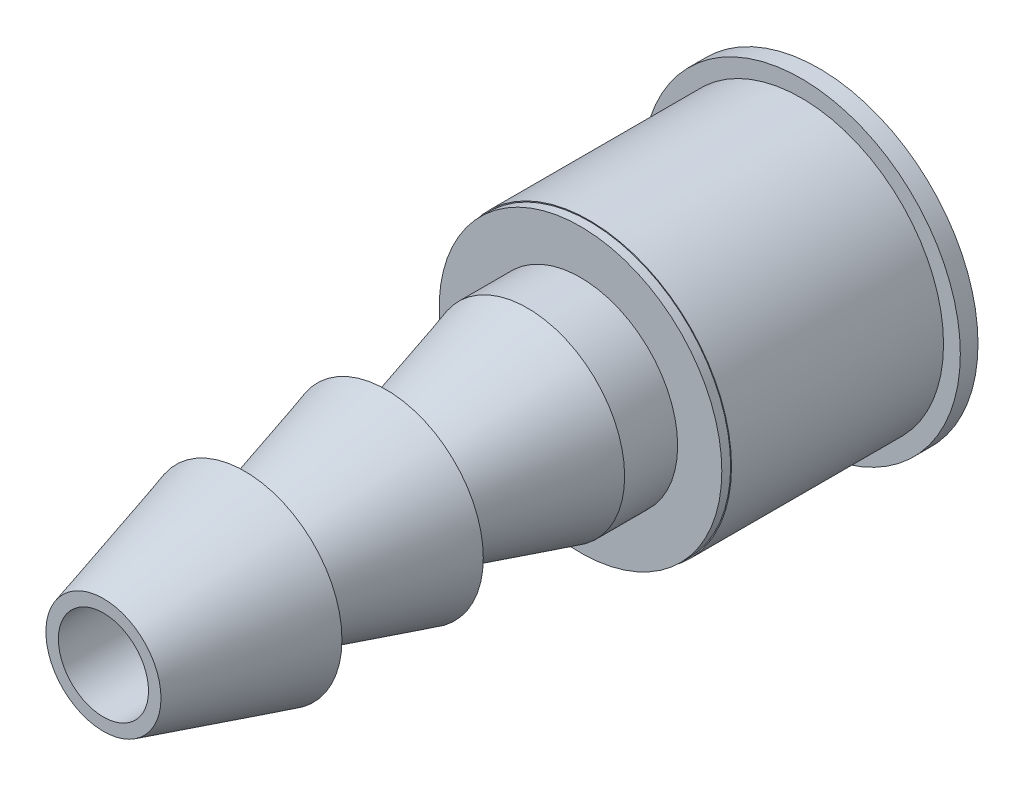
ISO-10303-21;
HEADER;
FILE_DESCRIPTION(('STEP AP214'),'2;1');
FILE_NAME('part.step','',(''),(''),'','','');
FILE_SCHEMA(('AUTOMOTIVE_DESIGN { 1 0 10303 214 1 1 1 1 }'));
ENDSEC;
DATA;
#1=APPLICATION_CONTEXT('core data for automotive mechanical design processes');
#2=APPLICATION_PROTOCOL_DEFINITION('international standard','automotive_design',2000,#1);
#3=PRODUCT_CONTEXT('',#1,'mechanical');
#4=PRODUCT('Part','Part','',(#3));
#5=PRODUCT_RELATED_PRODUCT_CATEGORY('part','',(#4));
#6=PRODUCT_DEFINITION_FORMATION('','',#4);
#7=PRODUCT_DEFINITION_CONTEXT('part definition',#1,'design');
#8=PRODUCT_DEFINITION('design','',#6,#7);
#9=PRODUCT_DEFINITION_SHAPE('','',#8);
#10=(LENGTH_UNIT() NAMED_UNIT(*) SI_UNIT(.MILLI.,.METRE.));
#11=(NAMED_UNIT(*) PLANE_ANGLE_UNIT() SI_UNIT($,.RADIAN.));
#12=(NAMED_UNIT(*) SI_UNIT($,.STERADIAN.) SOLID_ANGLE_UNIT());
#13=UNCERTAINTY_MEASURE_WITH_UNIT(LENGTH_MEASURE(1.E-05),#10,'distance_accuracy_value','');
#14=(GEOMETRIC_REPRESENTATION_CONTEXT(3) GLOBAL_UNCERTAINTY_ASSIGNED_CONTEXT((#13)) GLOBAL_UNIT_ASSIGNED_CONTEXT((#10,
#11,#12)) REPRESENTATION_CONTEXT('',''));
#15=CARTESIAN_POINT('',(0.,0.,0.));
#16=DIRECTION('',(0.,0.,1.));
#17=DIRECTION('',(1.,0.,0.));
#18=AXIS2_PLACEMENT_3D('',#15,#16,#17);
#19=CARTESIAN_POINT('',(0.,0.,1.));
#20=DIRECTION('',(0.,0.,-1.));
#21=DIRECTION('',(-1.,0.,0.));
#22=AXIS2_PLACEMENT_3D('',#19,#20,#21);
#23=CYLINDRICAL_SURFACE('',#22,9.);
#24=CARTESIAN_POINT('',(0.,0.,1.));
#25=DIRECTION('',(0.,0.,1.));
#26=DIRECTION('',(1.,0.,0.));
#27=AXIS2_PLACEMENT_3D('',#24,#25,#26);
#28=CIRCLE('',#27,9.);
#29=CARTESIAN_POINT('',(9.,0.,1.));
#30=VERTEX_POINT('',#29);
#31=EDGE_CURVE('E66',#30,#30,#28,.T.);
#32=ORIENTED_EDGE('',*,*,#31,.F.);
#33=EDGE_LOOP('',(#32));
#34=FACE_BOUND('',#33,.T.);
#35=CARTESIAN_POINT('',(0.,0.,0.));
#36=DIRECTION('',(0.,0.,1.));
#37=DIRECTION('',(1.,0.,0.));
#38=AXIS2_PLACEMENT_3D('',#35,#36,#37);
#39=CIRCLE('',#38,9.);
#40=CARTESIAN_POINT('',(9.,0.,0.));
#41=VERTEX_POINT('',#40);
#42=EDGE_CURVE('E70',#41,#41,#39,.T.);
#43=ORIENTED_EDGE('',*,*,#42,.T.);
#44=EDGE_LOOP('',(#43));
#45=FACE_BOUND('',#44,.T.);
#46=ADVANCED_FACE('F43',(#34,#45),#23,.T.);
#47=CARTESIAN_POINT('',(0.,0.,1.));
#48=DIRECTION('',(0.,0.,1.));
#49=DIRECTION('',(1.,0.,0.));
#50=AXIS2_PLACEMENT_3D('',#47,#48,#49);
#51=PLANE('',#50);
#52=CARTESIAN_POINT('',(0.,0.,1.));
#53=DIRECTION('',(0.,0.,1.));
#54=DIRECTION('',(1.,0.,0.));
#55=AXIS2_PLACEMENT_3D('',#52,#53,#54);
#56=CIRCLE('',#55,8.05);
#57=CARTESIAN_POINT('',(8.05,0.,1.));
#58=VERTEX_POINT('',#57);
#59=EDGE_CURVE('E54',#58,#58,#56,.T.);
#60=ORIENTED_EDGE('',*,*,#59,.F.);
#61=EDGE_LOOP('',(#60));
#62=FACE_BOUND('',#61,.T.);
#63=ORIENTED_EDGE('',*,*,#31,.T.);
#64=EDGE_LOOP('',(#63));
#65=FACE_BOUND('',#64,.T.);
#66=ADVANCED_FACE('F79',(#62,#65),#51,.T.);
#67=CARTESIAN_POINT('',(0.,0.,0.));
#68=DIRECTION('',(0.,0.,1.));
#69=DIRECTION('',(1.,0.,0.));
#70=AXIS2_PLACEMENT_3D('',#67,#68,#69);
#71=PLANE('',#70);
#72=CARTESIAN_POINT('',(0.,0.,0.));
#73=DIRECTION('',(0.,0.,-1.));
#74=DIRECTION('',(-1.,0.,0.));
#75=AXIS2_PLACEMENT_3D('',#72,#73,#74);
#76=CIRCLE('',#75,5.5);
#77=CARTESIAN_POINT('',(-5.5,0.,0.));
#78=VERTEX_POINT('',#77);
#79=EDGE_CURVE('E351',#78,#78,#76,.T.);
#80=ORIENTED_EDGE('',*,*,#79,.F.);
#81=EDGE_LOOP('',(#80));
#82=FACE_BOUND('',#81,.T.);
#83=ORIENTED_EDGE('',*,*,#42,.F.);
#84=EDGE_LOOP('',(#83));
#85=FACE_BOUND('',#84,.T.);
#86=ADVANCED_FACE('F77',(#82,#85),#71,.F.);
#87=CARTESIAN_POINT('',(0.,0.,13.));
#88=DIRECTION('',(0.,0.,-1.));
#89=DIRECTION('',(-1.,0.,0.));
#90=AXIS2_PLACEMENT_3D('',#87,#88,#89);
#91=CYLINDRICAL_SURFACE('',#90,8.05);
#92=CARTESIAN_POINT('',(0.,0.,13.));
#93=DIRECTION('',(0.,0.,1.));
#94=DIRECTION('',(1.,0.,0.));
#95=AXIS2_PLACEMENT_3D('',#92,#93,#94);
#96=CIRCLE('',#95,8.05);
#97=CARTESIAN_POINT('',(8.05,0.,13.));
#98=VERTEX_POINT('',#97);
#99=EDGE_CURVE('E65',#98,#98,#96,.T.);
#100=ORIENTED_EDGE('',*,*,#99,.F.);
#101=EDGE_LOOP('',(#100));
#102=FACE_BOUND('',#101,.T.);
#103=ORIENTED_EDGE('',*,*,#59,.T.);
#104=EDGE_LOOP('',(#103));
#105=FACE_BOUND('',#104,.T.);
#106=ADVANCED_FACE('F76',(#102,#105),#91,.T.);
#107=CARTESIAN_POINT('',(0.,0.,13.));
#108=DIRECTION('',(0.,0.,1.));
#109=DIRECTION('',(1.,0.,0.));
#110=AXIS2_PLACEMENT_3D('',#107,#108,#109);
#111=PLANE('',#110);
#112=CARTESIAN_POINT('',(0.,0.,13.));
#113=DIRECTION('',(0.,0.,1.));
#114=DIRECTION('',(1.,0.,0.));
#115=AXIS2_PLACEMENT_3D('',#112,#113,#114);
#116=CIRCLE('',#115,8.);
#117=CARTESIAN_POINT('',(8.,0.,13.));
#118=VERTEX_POINT('',#117);
#119=EDGE_CURVE('E49',#118,#118,#116,.T.);
#120=ORIENTED_EDGE('',*,*,#119,.F.);
#121=EDGE_LOOP('',(#120));
#122=FACE_BOUND('',#121,.T.);
#123=ORIENTED_EDGE('',*,*,#99,.T.);
#124=EDGE_LOOP('',(#123));
#125=FACE_BOUND('',#124,.T.);
#126=ADVANCED_FACE('F82',(#122,#125),#111,.T.);
#127=CARTESIAN_POINT('',(0.,0.,13.5));
#128=DIRECTION('',(0.,0.,-1.));
#129=DIRECTION('',(-1.,0.,0.));
#130=AXIS2_PLACEMENT_3D('',#127,#128,#129);
#131=CYLINDRICAL_SURFACE('',#130,8.);
#132=CARTESIAN_POINT('',(0.,0.,13.5));
#133=DIRECTION('',(0.,0.,1.));
#134=DIRECTION('',(1.,0.,0.));
#135=AXIS2_PLACEMENT_3D('',#132,#133,#134);
#136=CIRCLE('',#135,8.);
#137=CARTESIAN_POINT('',(8.,0.,13.5));
#138=VERTEX_POINT('',#137);
#139=EDGE_CURVE('E64',#138,#138,#136,.T.);
#140=ORIENTED_EDGE('',*,*,#139,.F.);
#141=EDGE_LOOP('',(#140));
#142=FACE_BOUND('',#141,.T.);
#143=ORIENTED_EDGE('',*,*,#119,.T.);
#144=EDGE_LOOP('',(#143));
#145=FACE_BOUND('',#144,.T.);
#146=ADVANCED_FACE('F124',(#142,#145),#131,.T.);
#147=CARTESIAN_POINT('',(0.,0.,13.5));
#148=DIRECTION('',(0.,0.,1.));
#149=DIRECTION('',(1.,0.,0.));
#150=AXIS2_PLACEMENT_3D('',#147,#148,#149);
#151=PLANE('',#150);
#152=CARTESIAN_POINT('',(0.,0.,13.5));
#153=DIRECTION('',(0.,0.,1.));
#154=DIRECTION('',(1.,0.,0.));
#155=AXIS2_PLACEMENT_3D('',#152,#153,#154);
#156=CIRCLE('',#155,5.5);
#157=CARTESIAN_POINT('',(5.5,0.,13.5));
#158=VERTEX_POINT('',#157);
#159=EDGE_CURVE('E10',#158,#158,#156,.T.);
#160=ORIENTED_EDGE('',*,*,#159,.F.);
#161=EDGE_LOOP('',(#160));
#162=FACE_BOUND('',#161,.T.);
#163=ORIENTED_EDGE('',*,*,#139,.T.);
#164=EDGE_LOOP('',(#163));
#165=FACE_BOUND('',#164,.T.);
#166=ADVANCED_FACE('F133',(#162,#165),#151,.T.);
#167=CARTESIAN_POINT('',(0.,0.,16.5));
#168=DIRECTION('',(0.,0.,-1.));
#169=DIRECTION('',(-1.,0.,0.));
#170=AXIS2_PLACEMENT_3D('',#167,#168,#169);
#171=CYLINDRICAL_SURFACE('',#170,5.5);
#172=CARTESIAN_POINT('',(0.,0.,16.5));
#173=DIRECTION('',(0.,0.,1.));
#174=DIRECTION('',(1.,0.,0.));
#175=AXIS2_PLACEMENT_3D('',#172,#173,#174);
#176=CIRCLE('',#175,5.5);
#177=CARTESIAN_POINT('',(5.5,0.,16.5));
#178=VERTEX_POINT('',#177);
#179=EDGE_CURVE('E56',#178,#178,#176,.T.);
#180=ORIENTED_EDGE('',*,*,#179,.F.);
#181=EDGE_LOOP('',(#180));
#182=FACE_BOUND('',#181,.T.);
#183=ORIENTED_EDGE('',*,*,#159,.T.);
#184=EDGE_LOOP('',(#183));
#185=FACE_BOUND('',#184,.T.);
#186=ADVANCED_FACE('F141',(#182,#185),#171,.T.);
#187=CARTESIAN_POINT('',(0.,0.,16.5));
#188=DIRECTION('',(0.,0.,-1.));
#189=DIRECTION('',(1.,0.,0.));
#190=AXIS2_PLACEMENT_3D('',#187,#188,#189);
#191=CONICAL_SURFACE('',#190,5.5,0.273318560862313);
#192=CARTESIAN_POINT('',(0.,0.,24.5));
#193=DIRECTION('',(0.,0.,1.));
#194=DIRECTION('',(1.,0.,0.));
#195=AXIS2_PLACEMENT_3D('',#192,#193,#194);
#196=CIRCLE('',#195,3.25732656296489);
#197=CARTESIAN_POINT('',(3.25732656296489,0.,24.5));
#198=VERTEX_POINT('',#197);
#199=EDGE_CURVE('E373',#198,#198,#196,.T.);
#200=ORIENTED_EDGE('',*,*,#199,.F.);
#201=EDGE_LOOP('',(#200));
#202=FACE_BOUND('',#201,.T.);
#203=ORIENTED_EDGE('',*,*,#179,.T.);
#204=EDGE_LOOP('',(#203));
#205=FACE_BOUND('',#204,.T.);
#206=ADVANCED_FACE('F153',(#202,#205),#191,.T.);
#207=CARTESIAN_POINT('',(0.,0.,24.5));
#208=DIRECTION('',(0.,0.,-1.));
#209=DIRECTION('',(1.,0.,0.));
#210=AXIS2_PLACEMENT_3D('',#207,#208,#209);
#211=CONICAL_SURFACE('',#210,5.5,0.273318560862313);
#212=CARTESIAN_POINT('',(0.,0.,32.5));
#213=DIRECTION('',(0.,0.,1.));
#214=DIRECTION('',(1.,0.,0.));
#215=AXIS2_PLACEMENT_3D('',#212,#213,#214);
#216=CIRCLE('',#215,3.25732656296489);
#217=CARTESIAN_POINT('',(3.25732656296489,0.,32.5));
#218=VERTEX_POINT('',#217);
#219=EDGE_CURVE('E371',#218,#218,#216,.T.);
#220=ORIENTED_EDGE('',*,*,#219,.F.);
#221=EDGE_LOOP('',(#220));
#222=FACE_BOUND('',#221,.T.);
#223=CARTESIAN_POINT('',(0.,0.,24.5));
#224=DIRECTION('',(0.,0.,1.));
#225=DIRECTION('',(1.,0.,0.));
#226=AXIS2_PLACEMENT_3D('',#223,#224,#225);
#227=CIRCLE('',#226,5.5);
#228=CARTESIAN_POINT('',(5.5,0.,24.5));
#229=VERTEX_POINT('',#228);
#230=EDGE_CURVE('E368',#229,#229,#227,.T.);
#231=ORIENTED_EDGE('',*,*,#230,.T.);
#232=EDGE_LOOP('',(#231));
#233=FACE_BOUND('',#232,.T.);
#234=ADVANCED_FACE('F162',(#222,#233),#211,.T.);
#235=CARTESIAN_POINT('',(0.,0.,24.5));
#236=DIRECTION('',(0.,0.,1.));
#237=DIRECTION('',(1.,0.,0.));
#238=AXIS2_PLACEMENT_3D('',#235,#236,#237);
#239=PLANE('',#238);
#240=ORIENTED_EDGE('',*,*,#199,.T.);
#241=EDGE_LOOP('',(#240));
#242=FACE_BOUND('',#241,.T.);
#243=ORIENTED_EDGE('',*,*,#230,.F.);
#244=EDGE_LOOP('',(#243));
#245=FACE_BOUND('',#244,.T.);
#246=ADVANCED_FACE('F175',(#242,#245),#239,.F.);
#247=CARTESIAN_POINT('',(0.,0.,32.5));
#248=DIRECTION('',(0.,0.,-1.));
#249=DIRECTION('',(1.,0.,0.));
#250=AXIS2_PLACEMENT_3D('',#247,#248,#249);
#251=CONICAL_SURFACE('',#250,5.5,0.273318560862313);
#252=CARTESIAN_POINT('',(0.,0.,40.5));
#253=DIRECTION('',(0.,0.,1.));
#254=DIRECTION('',(1.,0.,0.));
#255=AXIS2_PLACEMENT_3D('',#252,#253,#254);
#256=CIRCLE('',#255,3.25732656296489);
#257=CARTESIAN_POINT('',(3.25732656296489,0.,40.5));
#258=VERTEX_POINT('',#257);
#259=EDGE_CURVE('E362',#258,#258,#256,.T.);
#260=ORIENTED_EDGE('',*,*,#259,.F.);
#261=EDGE_LOOP('',(#260));
#262=FACE_BOUND('',#261,.T.);
#263=CARTESIAN_POINT('',(0.,0.,32.5));
#264=DIRECTION('',(0.,0.,1.));
#265=DIRECTION('',(1.,0.,0.));
#266=AXIS2_PLACEMENT_3D('',#263,#264,#265);
#267=CIRCLE('',#266,5.5);
#268=CARTESIAN_POINT('',(5.5,0.,32.5));
#269=VERTEX_POINT('',#268);
#270=EDGE_CURVE('E359',#269,#269,#267,.T.);
#271=ORIENTED_EDGE('',*,*,#270,.T.);
#272=EDGE_LOOP('',(#271));
#273=FACE_BOUND('',#272,.T.);
#274=ADVANCED_FACE('F185',(#262,#273),#251,.T.);
#275=CARTESIAN_POINT('',(0.,0.,40.5));
#276=DIRECTION('',(0.,0.,1.));
#277=DIRECTION('',(1.,0.,0.));
#278=AXIS2_PLACEMENT_3D('',#275,#276,#277);
#279=PLANE('',#278);
#280=CARTESIAN_POINT('',(0.,0.,40.5));
#281=DIRECTION('',(0.,0.,1.));
#282=DIRECTION('',(1.,0.,0.));
#283=AXIS2_PLACEMENT_3D('',#280,#281,#282);
#284=CIRCLE('',#283,2.55);
#285=CARTESIAN_POINT('',(2.55,0.,40.5));
#286=VERTEX_POINT('',#285);
#287=EDGE_CURVE('E46',#286,#286,#284,.T.);
#288=ORIENTED_EDGE('',*,*,#287,.F.);
#289=EDGE_LOOP('',(#288));
#290=FACE_BOUND('',#289,.T.);
#291=ORIENTED_EDGE('',*,*,#259,.T.);
#292=EDGE_LOOP('',(#291));
#293=FACE_BOUND('',#292,.T.);
#294=ADVANCED_FACE('F191',(#290,#293),#279,.T.);
#295=CARTESIAN_POINT('',(0.,0.,32.5));
#296=DIRECTION('',(0.,0.,1.));
#297=DIRECTION('',(1.,0.,0.));
#298=AXIS2_PLACEMENT_3D('',#295,#296,#297);
#299=PLANE('',#298);
#300=ORIENTED_EDGE('',*,*,#219,.T.);
#301=EDGE_LOOP('',(#300));
#302=FACE_BOUND('',#301,.T.);
#303=ORIENTED_EDGE('',*,*,#270,.F.);
#304=EDGE_LOOP('',(#303));
#305=FACE_BOUND('',#304,.T.);
#306=ADVANCED_FACE('F202',(#302,#305),#299,.F.);
#307=CARTESIAN_POINT('',(0.,0.,12.));
#308=DIRECTION('',(0.,0.,-1.));
#309=DIRECTION('',(-1.,0.,0.));
#310=AXIS2_PLACEMENT_3D('',#307,#308,#309);
#311=CYLINDRICAL_SURFACE('',#310,5.5);
#312=CARTESIAN_POINT('',(0.,0.,12.));
#313=DIRECTION('',(0.,0.,-1.));
#314=DIRECTION('',(-1.,0.,0.));
#315=AXIS2_PLACEMENT_3D('',#312,#313,#314);
#316=CIRCLE('',#315,5.5);
#317=CARTESIAN_POINT('',(-5.5,0.,12.));
#318=VERTEX_POINT('',#317);
#319=EDGE_CURVE('E357',#318,#318,#316,.T.);
#320=ORIENTED_EDGE('',*,*,#319,.F.);
#321=EDGE_LOOP('',(#320));
#322=FACE_BOUND('',#321,.T.);
#323=ORIENTED_EDGE('',*,*,#79,.T.);
#324=EDGE_LOOP('',(#323));
#325=FACE_BOUND('',#324,.T.);
#326=ADVANCED_FACE('F215',(#322,#325),#311,.F.);
#327=CARTESIAN_POINT('',(0.,0.,12.));
#328=DIRECTION('',(0.,0.,-1.));
#329=DIRECTION('',(-1.,0.,0.));
#330=AXIS2_PLACEMENT_3D('',#327,#328,#329);
#331=PLANE('',#330);
#332=CARTESIAN_POINT('',(0.,0.,12.));
#333=DIRECTION('',(0.,0.,-1.));
#334=DIRECTION('',(-1.,0.,0.));
#335=AXIS2_PLACEMENT_3D('',#332,#333,#334);
#336=CIRCLE('',#335,2.55);
#337=CARTESIAN_POINT('',(-2.55,0.,12.));
#338=VERTEX_POINT('',#337);
#339=EDGE_CURVE('E352',#338,#338,#336,.T.);
#340=ORIENTED_EDGE('',*,*,#339,.F.);
#341=EDGE_LOOP('',(#340));
#342=FACE_BOUND('',#341,.T.);
#343=ORIENTED_EDGE('',*,*,#319,.T.);
#344=EDGE_LOOP('',(#343));
#345=FACE_BOUND('',#344,.T.);
#346=ADVANCED_FACE('F224',(#342,#345),#331,.T.);
#347=CARTESIAN_POINT('',(0.,0.,50.));
#348=DIRECTION('',(0.,0.,-1.));
#349=DIRECTION('',(-1.,0.,0.));
#350=AXIS2_PLACEMENT_3D('',#347,#348,#349);
#351=CYLINDRICAL_SURFACE('',#350,2.55);
#352=ORIENTED_EDGE('',*,*,#287,.T.);
#353=EDGE_LOOP('',(#352));
#354=FACE_BOUND('',#353,.T.);
#355=ORIENTED_EDGE('',*,*,#339,.T.);
#356=EDGE_LOOP('',(#355));
#357=FACE_BOUND('',#356,.T.);
#358=ADVANCED_FACE('F233',(#354,#357),#351,.F.);
#359=CLOSED_SHELL('',(#46,#66,#86,#106,#126,#146,#166,#186,#206,#234,#246,#274,#294,#306,#326,
#346,#358));
#360=MANIFOLD_SOLID_BREP('B2',#359);
#361=ADVANCED_BREP_SHAPE_REPRESENTATION('',(#18,#360),#14);
#362=SHAPE_DEFINITION_REPRESENTATION(#9,#361);
ENDSEC;
END-ISO-10303-21;
